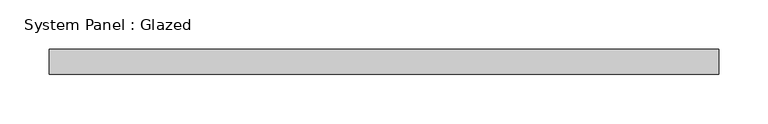
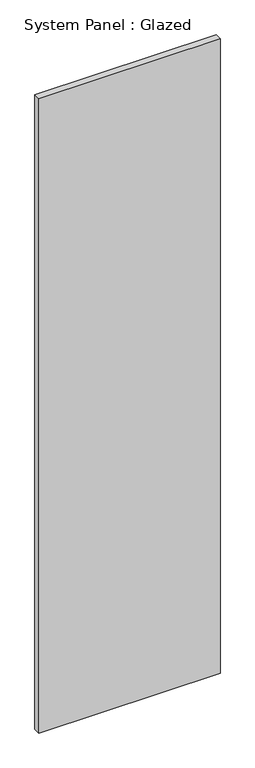
"""IFC4 building model written with IfcOpenShell, lengths in millimetres: plate geometry, System Panel : Glazed."""

from ifc_helpers import new_model, si_unit, origin, origin_with_axes, place, context, project, spatial, polyline, outline, extrude, source, transform, mapped, element, save


def system_panel_glazed_6ccdd28e(model_context):
    return source(origin(), model_context, "Body", "SweptSolid", [
        extrude(outline(polyline([(339.7250022, 19.05), (-339.7250022, 19.05), (-339.7250022, 44.45), (339.7250022, 44.45), (339.7250022, 19.05)])), origin_with_axes(), (0.0, 0.0, 1.0), 2514.6),
    ])


if __name__ == "__main__":
    model = new_model("IFC4")
    model_context = context("Model", 3, world=origin())
    ifc_project = project(units=[si_unit("LENGTHUNIT", "METRE", prefix="MILLI")], contexts=[model_context])
    site = spatial("IfcSite", under=ifc_project)
    building = spatial("IfcBuilding", under=site)
    placement = place(None, origin())
    system_panel_glazed_shape = system_panel_glazed_6ccdd28e(model_context)
    element("IfcPlate", 1, ObjectType="System Panel : Glazed", at=placement, inside=building, context=model_context, shape_type="MappedRepresentation", body=[
        mapped(system_panel_glazed_shape, transform((0.0, 0.0, 0.0), x_axis=(1.0, 0.0, 0.0), y_axis=(0.0, 1.0, 0.0), z_axis=(0.0, 0.0, 1.0))),
    ])
    save(model, "model.ifc")

# Revit data of these elements
# Type "System Panel : Glazed"
#   Construction Type Id = "GSP4R"
#   Analytic Construction = "1/8 in Pilkington single glazing"
#   Visual Light Transmittance = 0.9
#   Solar Heat Gain Coefficient = 0.86
#   Heat Transfer Coefficient (U) = 1.18115 BTU/(h·ft²·°F)
#   Define Thermal Properties by = 1
# Element 1 (IfcPlate, "System Panel : Glazed")
#   Materials on its faces: "Glass"
# Materials
#   "Glass": class "Glass", colour RGB 0 128 192, transparency 0.75, Description = "Soda Lime Glass", Cost = 0
